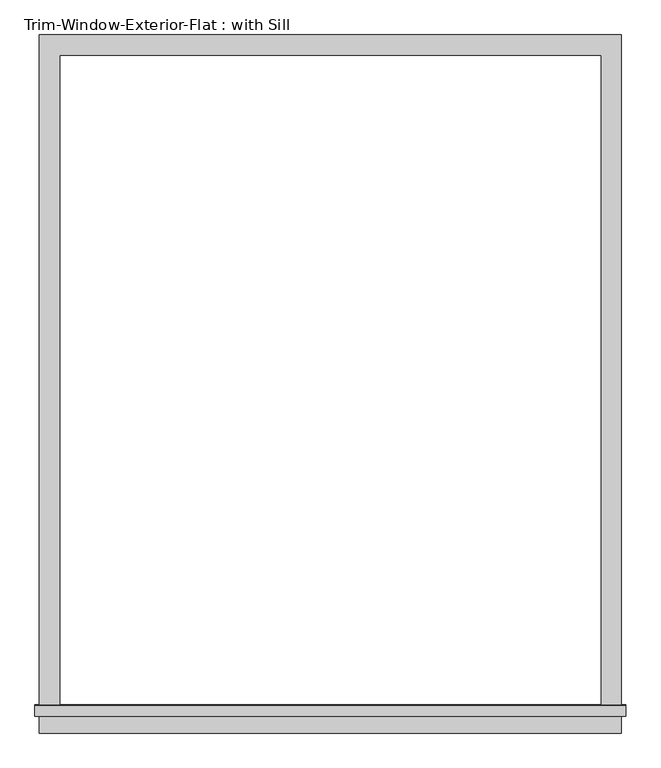
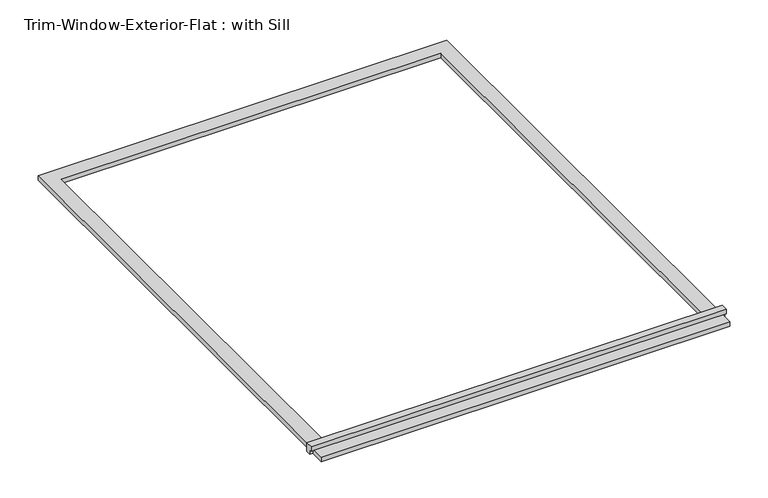
"""IFC4 building model written with IfcOpenShell, lengths in millimetres: proxy geometry, Trim-Window-Exterior-Flat : with Sill."""

from ifc_helpers import new_model, si_unit, frame, origin, origin_with_axes, place, context, project, spatial, polyline, outline, extrude, source, transform, mapped, element, save


def trim_window_exterior_flat_with_sill_698ed857(model_context):
    return source(origin(), model_context, "Body", "SweptSolid", [
        extrude(outline(polyline([(819.15, -1850.9823709), (819.15, -1908.1323709), (-819.15, -1908.1323709), (-819.15, -1850.9823709), (819.15, -1850.9823709)])), origin_with_axes(), (0.0, 0.0, 1.0), 19.05),
        extrude(outline(polyline([(-1860.55, 38.1), (-1831.2580645, 38.1), (-1828.8, 19.05), (-1828.8, 0.0), (-1850.9823709, 0.0), (-1850.9823709, 19.05), (-1860.55, 19.05), (-1860.55, 38.1)])), frame((-831.85, 0.0, 0.0), z_axis=(1.0, 0.0, 0.0), x_axis=(0.0, 1.0, 0.0)), (0.0, 0.0, 1.0), 1663.7),
        extrude(outline(polyline([(-819.15, 57.15), (819.15, 57.15), (819.15, -1828.8), (762.0, -1828.8), (762.0, 0.0), (-762.0, 0.0), (-762.0, -1828.8), (-819.15, -1828.8), (-819.15, 57.15)])), origin_with_axes(), (0.0, 0.0, 1.0), 19.05),
    ])


if __name__ == "__main__":
    model = new_model("IFC4")
    model_context = context("Model", 3, world=origin())
    ifc_project = project(units=[si_unit("LENGTHUNIT", "METRE", prefix="MILLI")], contexts=[model_context])
    site = spatial("IfcSite", under=ifc_project)
    building = spatial("IfcBuilding", under=site)
    placement = place(None, origin())
    trim_window_exterior_flat_with_sill_shape = trim_window_exterior_flat_with_sill_698ed857(model_context)
    element("IfcBuildingElementProxy", 1, Name="Trim-Window-Exterior-Flat : with Sill", ObjectType="Trim-Window-Exterior-Flat : with Sill", at=placement, inside=building, context=model_context, shape_type="MappedRepresentation", body=[
        mapped(trim_window_exterior_flat_with_sill_shape, transform((0.0, 0.0, 0.0), x_axis=(1.0, 0.0, 0.0), y_axis=(0.0, 1.0, 0.0), z_axis=(0.0, 0.0, 1.0))),
    ])
    save(model, "model.ifc")

# Revit data of these elements
# Type "Trim-Window-Exterior-Flat : with Sill"
#   Trim Width = 0' - 2 1/4"
#   Trim Thickness_Picture Frame = 0' - 1 1/4"
#   Trim Thickness_with Sill = 0' - 0 3/4"
#   Sill Thickness = 0' - 1 1/4"
#   Opening Width [instance default] = 2' - 0"
#   Opening Height [instance default] = 3' - 0"
#   Default Elevation = 4' - 0"
#   Sill = yes
#   Picture Frame = no
#   Trim Material [instance default] = none
# Element 1 (IfcBuildingElementProxy, "Trim-Window-Exterior-Flat : with Sill")
#   Opening Width = 5' - 0"
#   Opening Height = 6' - 0"
#   Trim Material = Clad - White
#   Materials on its faces: "Clad - White"
# Materials
#   "Clad - White": class "Wood", colour RGB 242 242 238, transparency 0, Cost = 0
